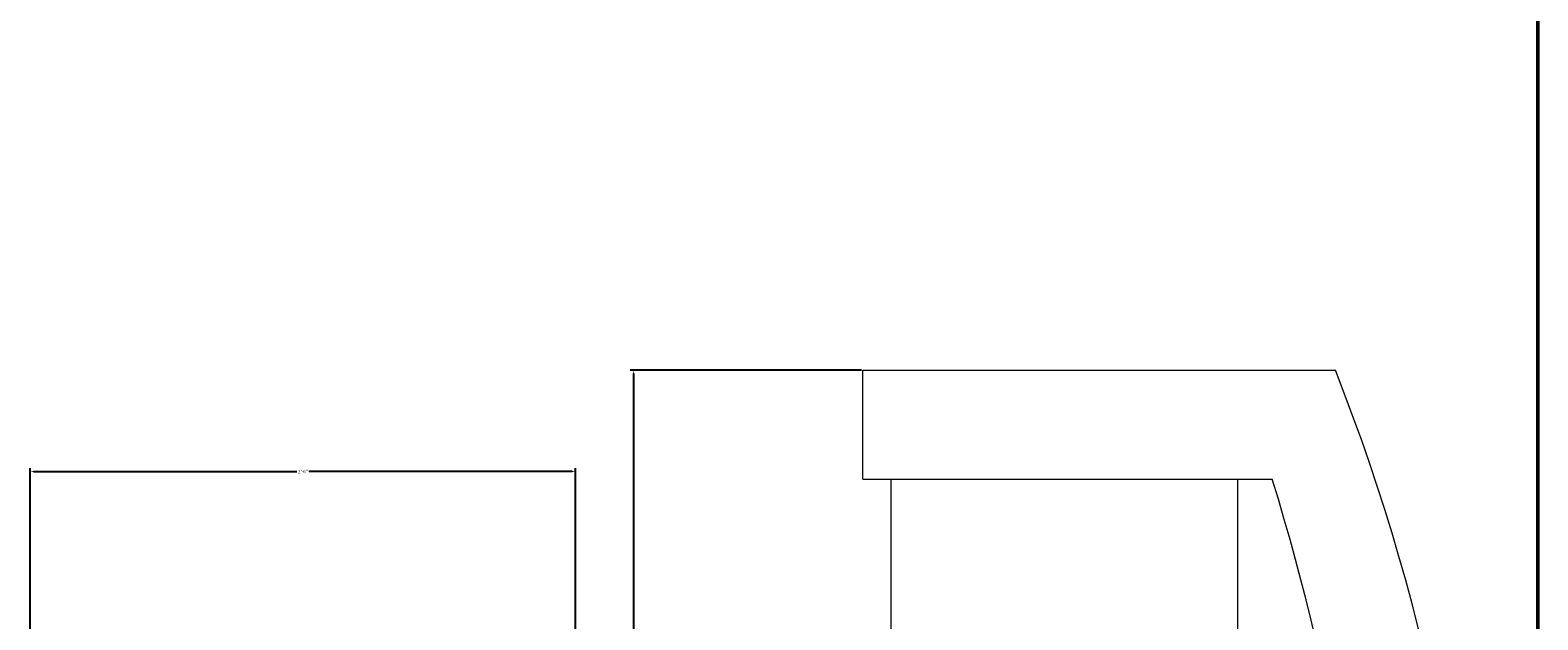
# Model space of a CAD drawing. Units: inches. Extents: x -105 to 1196, y -792 to 119.
# Tile 16 of 23: x 232 to 315, y -318 to -285. Entities that reach past the tile are written whole.
import ezdxf

# ---------------------------------------------------------------- set-up
doc = ezdxf.new("R2010")
doc.units = ezdxf.units.IN
doc.header["$MEASUREMENT"] = 0
for name, color, linetype, lineweight in [('A-ANNO-DIMS', 2, 'Continuous', 18), ('A-FURN', 8, 'Continuous', 18), ('A-WALL', 3, 'Continuous', 50)]:
    doc.layers.add(name, color=color, linetype=linetype, lineweight=lineweight)
doc.styles.get("Standard").update_dxf_attribs({"font": 'arial.ttf'})
doc.dimstyles.get("Standard").update_dxf_attribs({"dimtxt": 0.18, "dimasz": 0.18, "dimexe": 0.18, "dimexo": 0.0625, "dimgap": 0.09, "dimtad": 0, "dimtih": 1, "dimtoh": 1, "dimdec": 1, "dimzin": 0, "dimdsep": 46, "dimlunit": 4, "dimtxsty": 'Standard', "dimcen": 0.09, "dimadec": 0, "dimazin": 0, "dimtfac": 1, "dimtdec": 1, "dimtofl": 0, "dimtmove": 0, "dimatfit": 3, "dimfxl": 1, "dimtolj": 1, "dimtzin": 0, "dimarcsym": 0})

# ---------------------------------------------------------------- blocks, each defined once
blk = doc.blocks.new('Sofa - Roundback 7 ft.')
for p, q in [((-12.00002, -32.4421), (-12.00003, -6.5971)), ((11.99997, -32.4421), (11.99998, -6.5971)), ((-36.000027, -34), (-36.000027, -11.4696)), ((35.99998, -34), (35.99998, -11.4696)), ((-35.999844, -13.3819), (35.9998, -13.3819)), ((-36.000027, -32.4421), (35.99998, -32.4421))]:
    blk.add_line(p, q)
for points in [[(-36.000027, -34), (-42.000027, -34), (-42.000027, -8)], [(41.99998, -8), (41.99998, -34), (35.99998, -34)]]:
    blk.add_lwpolyline(points)
for centre, radius, start, end in [((0, -114.25), 114.25, 68.43141, 111.5686), ((-0.00001, -127.1968), 121.1968, 72.72033, 107.2797)]:
    blk.add_arc(centre, radius, start, end)
blk = doc.blocks.new('*D77')
at = {"layer": 'A-ANNO-DIMS', "color": 0, "lineweight": -2, "transparency": 16777216}
for p, q in [((277.544, -304.122), (264.827, -304.122)), ((265.007, -304.302), (265.007, -345.939)), ((265.007, -387.942), (265.007, -346.305)), ((277.544, -388.122), (264.827, -388.122))]:
    blk.add_line(p, q, dxfattribs=at)
at = {"layer": 'A-ANNO-DIMS', "color": 0, "transparency": 16777216}
for points in [[(264.977, -304.302), (265.037, -304.302), (265.007, -304.122)], [(264.977, -387.942), (265.037, -387.942), (265.007, -388.122)]]:
    blk.add_solid(points, dxfattribs=at)
at = {"layer": 'Defpoints', "color": 0, "transparency": 16777216}
for p in [(277.607, -304.122), (265.007, -388.122), (277.607, -388.122)]:
    blk.add_point(p, dxfattribs=at)
at = {"layer": 'A-ANNO-DIMS', "color": 0, "transparency": 16777216, "insert": (265.007, -346.122), "char_height": 0.18, "attachment_point": 5}
blk.add_mtext('\\A1;SOFA 7\'-0"', dxfattribs=at)
blk = doc.blocks.new('*D84')
at = {"layer": 'A-ANNO-DIMS', "color": 0, "lineweight": -2, "transparency": 16777216}
for p, q in [((231.815, -318.633), (231.815, -309.515)), ((231.995, -309.695), (246.484, -309.695)), ((261.635, -309.695), (247.146, -309.695)), ((261.815, -318.633), (261.815, -309.515))]:
    blk.add_line(p, q, dxfattribs=at)
at = {"layer": 'A-ANNO-DIMS', "color": 0, "transparency": 16777216}
for points in [[(231.995, -309.665), (231.995, -309.725), (231.815, -309.695)], [(261.635, -309.665), (261.635, -309.725), (261.815, -309.695)]]:
    blk.add_solid(points, dxfattribs=at)
at = {"layer": 'Defpoints', "color": 0, "transparency": 16777216}
for p in [(231.815, -309.695), (231.815, -318.695), (261.815, -318.695)]:
    blk.add_point(p, dxfattribs=at)
at = {"layer": 'A-ANNO-DIMS', "color": 0, "transparency": 16777216, "insert": (246.815, -309.695), "char_height": 0.18, "attachment_point": 5}
blk.add_mtext('\\A1;2\'-6"', dxfattribs=at)

msp = doc.modelspace()

# ---------------------------------------------------------------- linework, layer by layer
at = {"layer": 'A-WALL'}
msp.add_line((314.744, -268.115), (314.744, -429.227), dxfattribs=at)

# ---------------------------------------------------------------- block references
at = {"layer": 'A-FURN', "rotation": 270}
msp.add_blockref('Sofa - Roundback 7 ft.', (311.607, -346.122), dxfattribs=at)

# ---------------------------------------------------------------- dimensions: what is measured, and where the dimension line sits
at = {"layer": 'A-ANNO-DIMS'}
dim = msp.add_linear_dim(base=(265.007, -388.122), p1=(277.607, -304.122), p2=(277.607, -388.122), angle=270, text='SOFA <>', dimstyle='Standard', override={"dimdec": 1, "dimlfac": 1, "dimrnd": 0, "dimzin": 1, "dimdsep": 46, "dimlunit": 4, "dimfrac": 2}, dxfattribs=at)
dim.commit()
dim.dimension.update_dxf_attribs({"geometry": '*D77', "text_midpoint": (265.007, -346.122)})
dim = msp.add_linear_dim(base=(231.815, -309.695), p1=(261.815, -318.695), p2=(231.815, -318.695), angle=180, dimstyle='Standard', override={"dimdec": 1, "dimlfac": 1, "dimrnd": 0, "dimzin": 1, "dimdsep": 46, "dimlunit": 4, "dimfrac": 2}, dxfattribs=at)
dim.commit()
dim.dimension.update_dxf_attribs({"geometry": '*D84', "text_midpoint": (246.815, -309.695)})

doc.saveas('drawing.dxf')
